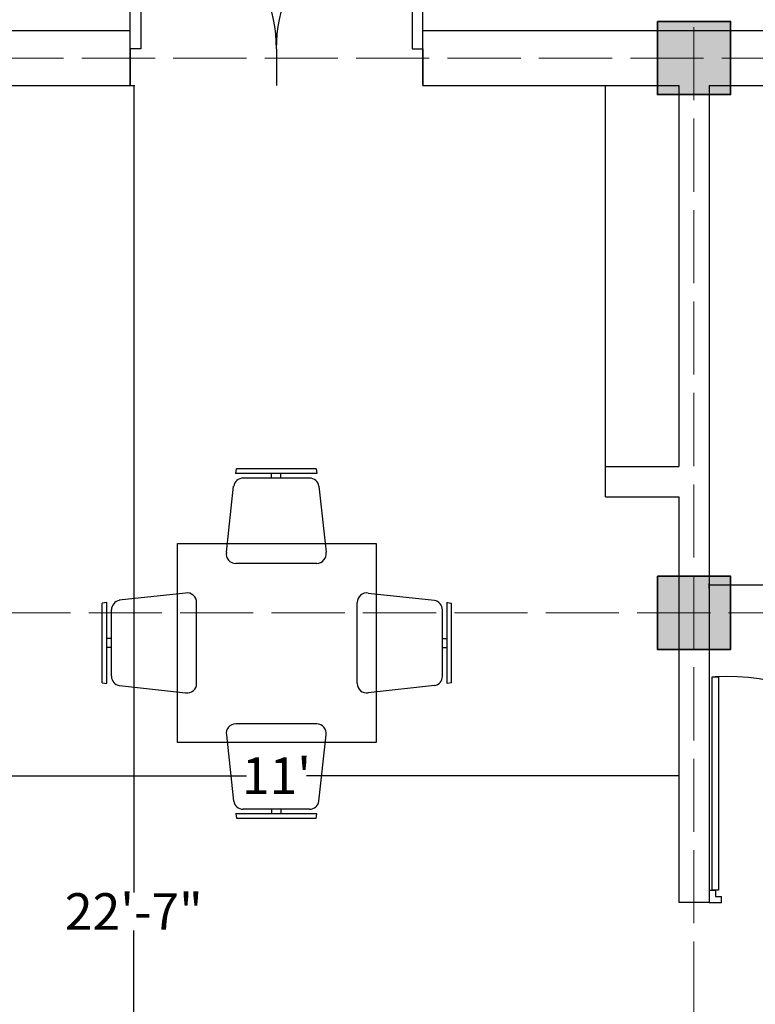
# Model space of a CAD drawing. Units: inches. Extents: x -113 to 5399, y -1393 to 3302.
# Tile 8 of 40: x 1073 to 1194, y 627 to 788. Entities that reach past the tile are written whole.
import ezdxf

# ---------------------------------------------------------------- set-up
doc = ezdxf.new("R2010")
doc.units = ezdxf.units.IN
doc.header["$MEASUREMENT"] = 0
doc.linetypes.add('ACAD_ISO02W100', pattern=[15, 12, -3])
for name, color, linetype, lineweight in [('A-ANNO-DIMS', 254, 'Continuous', 18), ('A-COLS', 7, 'Continuous', 35), ('doors', 2, 'Continuous', 25), ('furniture', 131, 'Continuous', 18), ('GRIDS', 7, 'ACAD_ISO02W100', 13), ('walls', 1, 'Continuous', 25)]:
    doc.layers.add(name, color=color, linetype=linetype, lineweight=lineweight)
doc.layers.add('B-FURNITURE', color=22, linetype='Continuous')
doc.styles.get("Standard").update_dxf_attribs({"font": 'arial.ttf'})
doc.dimstyles.get("Standard").update_dxf_attribs({"dimtxt": 6, "dimasz": 0.18, "dimexe": 0.18, "dimexo": 0.0625, "dimgap": 0.09, "dimtad": 0, "dimtih": 1, "dimtoh": 1, "dimdec": 1, "dimzin": 0, "dimdsep": 46, "dimlunit": 4, "dimtxsty": 'Standard', "dimblk": 'ARCHTICK', "dimcen": 0.09, "dimadec": 0, "dimazin": 0, "dimtfac": 1, "dimtdec": 1, "dimtofl": 0, "dimtmove": 0, "dimatfit": 3, "dimfxl": 1, "dimtolj": 1, "dimtzin": 0, "dimarcsym": 0})

# ---------------------------------------------------------------- blocks, each defined once
blk = doc.blocks.new('A$C6ACA79D1')
at = {"layer": 'B-FURNITURE'}
for p, q in [((-0.5034, 0.0535), (-0.8012, -0.2442)), ((-0.5034, 0.0535), (-0.4835, 0.0392)), ((0.4842, 0.0434), (0.5041, 0.0577)), ((0.8012, -0.239), (0.5034, 0.0587)), ((-0.4835, 0.0392), (-0.7869, -0.2642)), ((-0.4291, 0.0003), (-0.1547, -0.2204)), ((0.7869, -0.259), (0.4835, 0.0444)), ((0.7427, -0.249), (0.4935, 0.0002)), ((-0.4935, -0.005), (-0.7427, -0.2542)), ((-0.601, -0.1125), (-0.6181, -0.0954)), ((0.601, -0.1073), (0.6181, -0.0902)), ((-0.6352, -0.1467), (-0.6523, -0.1296)), ((0.6352, -0.1415), (0.6523, -0.1244)), ((-0.7859, -0.2635), (-0.8002, -0.2436)), ((0.8012, -0.239), (0.7869, -0.259)), ((-0.1485, -0.2964), (-0.4513, -0.5992)), ((0.4513, -0.594), (0.1485, -0.2912)), ((0.748, -0.3133), (0.5273, -0.5877)), ((-0.1485, -1.1937), (-0.4513, -0.8909)), ((0.4513, -0.8961), (0.1485, -1.199)), ((0.748, -1.1768), (0.5273, -0.9024)), ((-0.5034, -1.5436), (-0.8012, -1.2459)), ((-0.7859, -1.2266), (-0.8002, -1.2466)), ((-0.4835, -1.5293), (-0.7869, -1.226)), ((-0.4935, -1.4851), (-0.7427, -1.236)), ((0.7869, -1.2312), (0.4835, -1.5346)), ((0.7427, -1.2412), (0.4935, -1.4903)), ((0.8012, -1.2511), (0.7869, -1.2312)), ((-0.4291, -1.4904), (-0.1547, -1.2698)), ((0.8012, -1.2511), (0.5034, -1.5488)), ((-0.6352, -1.3434), (-0.6523, -1.3605)), ((0.6352, -1.3486), (0.6523, -1.3657)), ((-0.601, -1.3776), (-0.6181, -1.3948)), ((0.601, -1.3829), (0.6181, -1.4)), ((-0.5034, -1.5436), (-0.4835, -1.5293)), ((0.4842, -1.5336), (0.5041, -1.5478))]:
    blk.add_line(p, q, dxfattribs=at)
at = {"layer": 'B-FURNITURE', "ltscale": 300}
for p, q in [((0.1547, -0.2152), (0.4291, 0.0055)), ((-0.5273, -0.593), (-0.748, -0.3186)), ((-0.5273, -0.8972), (-0.748, -1.1716)), ((0.1547, -1.275), (0.4291, -1.4956))]:
    blk.add_line(p, q, dxfattribs=at)
blk.add_lwpolyline([(-0.7425, -0.7425), (0, 0), (0.7425, -0.7425), (0, -1.4849)], close=True, dxfattribs=at)
at = {"layer": 'B-FURNITURE', "ltscale": 400}
for centre, start, end in [((-0.4582, -0.0403), 54.4069, 135), ((0.4589, -0.0361), 45, 125.5931), ((-0.7063, -0.2888), 135, 215.5931), ((0.7073, -0.2843), 324.4069, 45), ((-0.7063, -1.2013), 144.4069, 225), ((0.7073, -1.2059), 315, 35.5931), ((-0.4582, -1.4498), 225, 305.5931), ((0.4589, -1.454), 234.4069, 315)]:
    blk.add_arc(centre, 0.0499, start, end, dxfattribs=at)
at = {"layer": 'B-FURNITURE', "ltscale": 300}
for centre, start, end in [((-0.1838, -0.261), 315, 54.4069), ((0.1838, -0.2558), 125.5931, 225), ((-0.4866, -0.5639), 215.5931, 315), ((0.4866, -0.5586), 225, 324.4069), ((-0.4866, -0.9263), 45, 144.4069), ((0.4866, -0.9315), 35.5931, 135), ((-0.1838, -1.2291), 305.5931, 45), ((0.1838, -1.2343), 135, 234.4069)]:
    blk.add_arc(centre, 0.05, start, end, dxfattribs=at)
blk = doc.blocks.new('*U2')
for p, q in [((0, 0), (0, -6)), ((24, 0), (24, -6))]:
    blk.add_line(p, q)
blk.add_lwpolyline([(0, 0), (0, 24), (1.75, 24), (1.75, 0)], close=True)
blk.add_arc((0, 0), 24, 0, 90)
blk = doc.blocks.new('_ArchTick')
at = {"color": 0, "linetype": 'ByBlock', "const_width": 0.15}
blk.add_lwpolyline([(-0.5, -0.5), (0.5, 0.5)], dxfattribs=at)
blk = doc.blocks.new('*D25')
at = {"layer": 'A-ANNO-DIMS', "color": 0, "lineweight": -2, "transparency": 16777216}
for p, q in [((1091.29, 777.53), (1092, 777.53)), ((1091.82, 777.53), (1091.82, 645.13)), ((1091.82, 506.53), (1091.82, 638.93)), ((1093.84, 506.53), (1091.64, 506.53))]:
    blk.add_line(p, q, dxfattribs=at)
at = {"layer": 'Defpoints', "color": 0, "transparency": 16777216}
for p in [(1091.23, 777.53), (1091.82, 777.53), (1093.91, 506.53)]:
    blk.add_point(p, dxfattribs=at)
at = {"layer": 'A-ANNO-DIMS', "color": 0, "lineweight": -2, "transparency": 16777216, "xscale": 0.18, "yscale": 0.18, "zscale": 0.18}
for p, rotation in [((1091.82, 777.53), 90), ((1091.82, 506.53), 270)]:
    blk.add_blockref('_ArchTick', p, dxfattribs=dict(at, rotation=rotation))
at = {"layer": 'A-ANNO-DIMS', "color": 0, "transparency": 16777216, "insert": (1091.82, 642.03), "char_height": 6, "attachment_point": 5}
blk.add_mtext('\\A1;22\'-7"', dxfattribs=at)
blk = doc.blocks.new('*D26')
at = {"layer": 'A-ANNO-DIMS', "color": 0, "lineweight": -2, "transparency": 16777216}
for p, q in [((1049.23, 664.47), (1049.23, 664.12)), ((1049.23, 664.3), (1110.33, 664.3)), ((1181.23, 664.3), (1120.13, 664.3)), ((1181.23, 664.47), (1181.23, 664.12))]:
    blk.add_line(p, q, dxfattribs=at)
at = {"layer": 'Defpoints', "color": 0, "transparency": 16777216}
for p in [(1049.23, 664.53), (1181.23, 664.53), (1181.23, 664.3)]:
    blk.add_point(p, dxfattribs=at)
at = {"layer": 'A-ANNO-DIMS', "color": 0, "lineweight": -2, "transparency": 16777216, "xscale": 0.18, "yscale": 0.18, "zscale": 0.18, "rotation": 180}
blk.add_blockref('_ArchTick', (1049.23, 664.3), dxfattribs=at)
at = {"layer": 'A-ANNO-DIMS', "color": 0, "lineweight": -2, "transparency": 16777216, "xscale": 0.18, "yscale": 0.18, "zscale": 0.18}
blk.add_blockref('_ArchTick', (1181.23, 664.3), dxfattribs=at)
at = {"layer": 'A-ANNO-DIMS', "color": 0, "transparency": 16777216, "insert": (1115.23, 664.3), "char_height": 6, "attachment_point": 5}
blk.add_mtext("\\A1;11'", dxfattribs=at)
blk = doc.blocks.new('*D40')
at = {"layer": 'A-ANNO-DIMS', "color": 0, "lineweight": -2, "transparency": 16777216}
for p, q in [((1186.23, 695), (1186.23, 695.81)), ((1186.23, 695.63), (1247.33, 695.63)), ((1318.23, 695.63), (1257.13, 695.63)), ((1318.23, 695), (1318.23, 695.81))]:
    blk.add_line(p, q, dxfattribs=at)
at = {"layer": 'Defpoints', "color": 0, "transparency": 16777216}
for p in [(1186.23, 695.63), (1186.23, 694.94), (1318.23, 694.94)]:
    blk.add_point(p, dxfattribs=at)
at = {"layer": 'A-ANNO-DIMS', "color": 0, "lineweight": -2, "transparency": 16777216, "xscale": 0.18, "yscale": 0.18, "zscale": 0.18, "rotation": 180}
blk.add_blockref('_ArchTick', (1186.23, 695.63), dxfattribs=at)
at = {"layer": 'A-ANNO-DIMS', "color": 0, "lineweight": -2, "transparency": 16777216, "xscale": 0.18, "yscale": 0.18, "zscale": 0.18}
blk.add_blockref('_ArchTick', (1318.23, 695.63), dxfattribs=at)
at = {"layer": 'A-ANNO-DIMS', "color": 0, "transparency": 16777216, "insert": (1252.23, 695.63), "char_height": 6, "attachment_point": 5}
blk.add_mtext("\\A1;11'", dxfattribs=at)
blk = doc.blocks.new('COLUMN-12IN-SQUARE')
h = blk.add_hatch(color=256)
h.dxf.hatch_style = 1
h.paths.add_polyline_path([(6, 6), (-6, 6), (-6, -6), (6, -6)])
blk.add_lwpolyline([(-6, 6), (6, 6), (6, -6), (-6, -6)], close=True)
blk = doc.blocks.new('DOOR-SINGLE-36IN-PLAN')
for p, q in [((0.5, 2), (0.5, 36.98)), ((0.5, 36.98), (1.5, 36.98)), ((1.5, 36.98), (1.5, 2)), ((0, 2), (0, 0)), ((0, 2), (1.04, 2)), ((1.5, 2), (0.5, 2)), ((1.04, 2), (1.04, 0.98)), ((40, 2), (38.96, 2)), ((38.96, 2), (38.96, 0.98)), ((40, 0), (40, 2)), ((1.04, 0.98), (2, 0.98)), ((2, 0), (2, 0.98)), ((38.96, 0.98), (38, 0.98)), ((38, 0), (38, 0.98)), ((0, 0), (2, 0)), ((0, 0), (2, 0)), ((38, 0), (40, 0))]:
    blk.add_line(p, q)
blk.add_arc((2.94, 0.99), 36.04, 1.6003, 93.0893)

msp = doc.modelspace()

# ---------------------------------------------------------------- linework, layer by layer
at = {"layer": 'GRIDS'}
for p, q in [((1183.73, 922.09), (1183.73, 46.81)), ((768.3, 782.03), (1417.18, 782.03)), ((769.42, 691.03), (1426.54, 691.03))]:
    msp.add_line(p, q, dxfattribs=at)
at = {"layer": 'walls'}
for p, q in [((894.23, 786.53), (1091.23, 786.53)), ((1091.23, 777.53), (1091.23, 786.53)), ((1139.23, 777.53), (1139.23, 786.53)), ((1139.23, 786.53), (1186.23, 786.53)), ((1186.23, 786.53), (1327.23, 786.53)), ((1049.23, 777.53), (1091.23, 777.53)), ((1139.23, 777.53), (1181.23, 777.53)), ((1169.23, 715.03), (1169.23, 777.53)), ((1181.23, 777.53), (1181.23, 715.03)), ((1186.23, 777.53), (1186.23, 643.53)), ((1186.23, 777.53), (1318.23, 777.53)), ((1169.23, 715.03), (1181.23, 715.03)), ((1169.23, 710.03), (1169.23, 715.03)), ((1169.23, 710.03), (1181.23, 710.03)), ((1181.23, 710.03), (1181.23, 643.53)), ((1186.23, 643.53), (1181.23, 643.53))]:
    msp.add_line(p, q, dxfattribs=at)

# ---------------------------------------------------------------- block references
at = {"layer": 'A-COLS'}
for p in [(1183.73, 782.03), (1183.73, 691.03)]:
    msp.add_blockref('COLUMN-12IN-SQUARE', p, dxfattribs=at)
at = {"layer": 'doors'}
for name, p in [('*U2', (1091.23, 783.53)), ('DOOR-SINGLE-36IN-PLAN', (1186.23, 643.53))]:
    msp.add_blockref(name, p, dxfattribs=at)
at = {"layer": 'doors', "xscale": -1}
msp.add_blockref('*U2', (1139.23, 783.53), dxfattribs=at)
at = {"layer": 'furniture', "xscale": 31.0665876167328, "yscale": 31.0665876167328, "zscale": 31.0665876167328, "rotation": 314.9999999999397}
msp.add_blockref('A$C6ACA79D1', (1131.61, 702.39), dxfattribs=at)

# ---------------------------------------------------------------- dimensions: what is measured, and where the dimension line sits
at = {"layer": 'A-ANNO-DIMS'}
dim = msp.add_linear_dim(base=(1091.82, 777.53), p1=(1093.91, 506.53), p2=(1091.23, 777.53), angle=90, dimstyle='Standard', override={"dimclrd": 0, "dimclre": 0, "dimclrt": 0}, dxfattribs=at)
dim.commit()
dim.dimension.update_dxf_attribs({"geometry": '*D25', "text_midpoint": (1091.82, 642.03)})
for base, p1, p2, picture, middle in [((1186.23, 695.63), (1318.23, 694.94), (1186.23, 694.94), '*D40', (1252.23, 695.63)), ((1181.23, 664.3), (1049.23, 664.53), (1181.23, 664.53), '*D26', (1115.23, 664.3))]:
    dim = msp.add_linear_dim(base=base, p1=p1, p2=p2, dimstyle='Standard', override={"dimclrd": 0, "dimclre": 0, "dimclrt": 0}, dxfattribs=at)
    dim.commit()
    dim.dimension.update_dxf_attribs({"geometry": picture, "text_midpoint": middle})

doc.saveas('drawing.dxf')
